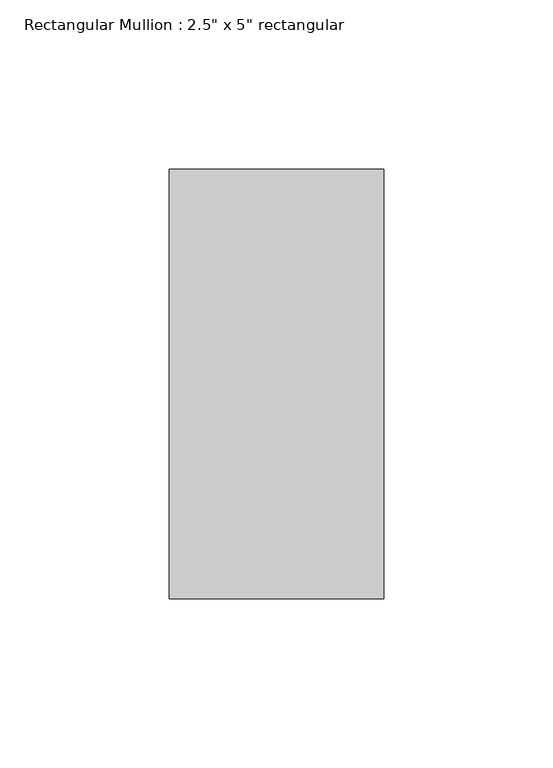
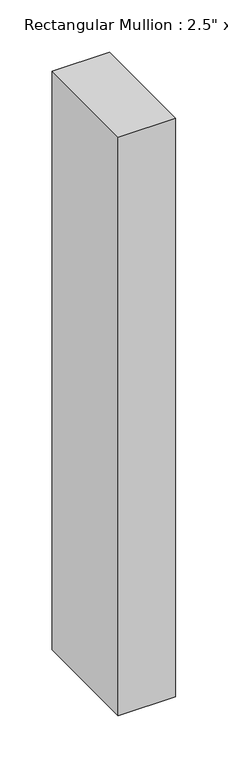
"""IFC4 building model written with IfcOpenShell, lengths in millimetres: member geometry."""

from ifc_helpers import new_model, si_unit, frame, origin, place, context, project, spatial, polyline, outline, extrude, source, transform, mapped, element, save


def member_819a76f2(model_context):
    return source(origin(), model_context, "Body", "SweptSolid", [
        extrude(outline(polyline([(0.0, 63.5), (0.0, -63.5), (-63.5, -63.5), (-63.5, 63.5), (0.0, 63.5)])), frame((0.0, 0.0, -677.019824), z_axis=(0.0, 0.0, 1.0), x_axis=(1.0, 0.0, 0.0)), (0.0, 0.0, 1.0), 677.019824),
    ])


if __name__ == "__main__":
    model = new_model("IFC4")
    model_context = context("Model", 3, world=origin())
    ifc_project = project(units=[si_unit("LENGTHUNIT", "METRE", prefix="MILLI")], contexts=[model_context])
    site = spatial("IfcSite", under=ifc_project)
    building = spatial("IfcBuilding", under=site)
    placement = place(None, origin())
    member_shape = member_819a76f2(model_context)
    element("IfcMember", 1, ObjectType="Rectangular Mullion : 2.5\" x 5\" rectangular", at=placement, inside=building, context=model_context, shape_type="MappedRepresentation", body=[
        mapped(member_shape, transform((0.0, 0.0, 0.0), x_axis=(1.0, 0.0, 0.0), y_axis=(0.0, 1.0, 0.0), z_axis=(0.0, 0.0, 1.0))),
    ])
    save(model, "model.ifc")

# Revit data of these elements
# Type "Rectangular Mullion : 2.5\" x 5\" rectangular"
#   built-in parameter 1007304 = 0.416667 (stored number, unit not read)
#   built-in parameter 1007301 = 0.104167 (stored number, unit not read)
#   built-in parameter 1007300 = 0.104167 (stored number, unit not read)
# Element 1 (IfcMember, "Rectangular Mullion : 2.5\" x 5\" rectangular")
#   Materials on its faces: "Aluminum"
# Materials
#   "Aluminum": class "Metal", colour RGB 247 247 247, transparency 0, Description = "Aluminum 6061", Cost = 0
